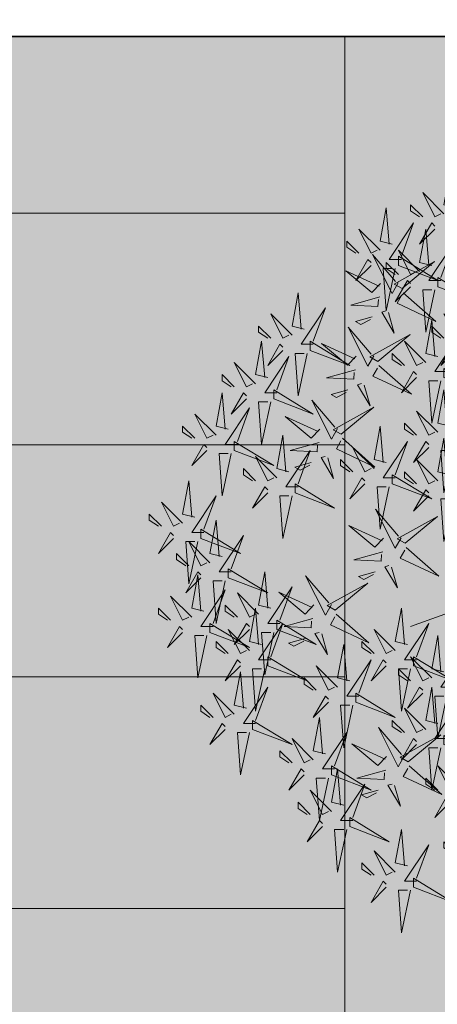
# Model space of a CAD drawing. Units: inches. Extents: x 1704 to 6393, y -157 to 1172.
# Tile 105 of 122: x 2654 to 2667, y 1002 to 1034. Entities that reach past the tile are written whole.
import ezdxf

# ---------------------------------------------------------------- set-up
doc = ezdxf.new("R2010")
doc.units = ezdxf.units.IN
doc.header["$MEASUREMENT"] = 0
for name, color, linetype, lineweight in [('A-ANNO-DIMS', 7, 'Continuous', 13), ('C-PROP', 7, 'Continuous', 35), ('L-DECK-PLNK-PATT', 250, 'Continuous', 13), ('L-HRDS', 8, 'Continuous', 18), ('L-shrub', 74, 'Continuous', 18)]:
    doc.layers.add(name, color=color, linetype=linetype, lineweight=lineweight)
doc.layers.add('L-DECK-PATT', color=35, linetype='Continuous', lineweight=13, true_color=0xa6725b)
doc.layers.add('L-HRDS-PATT', color=9, linetype='Continuous', lineweight=13, true_color=0xc5c1ba)
doc.styles.get("Standard").update_dxf_attribs({"font": 'arial.ttf'})
doc.dimstyles.get("Standard").update_dxf_attribs({"dimtxt": 6, "dimasz": 2, "dimexe": 0.18, "dimexo": 0.0625, "dimgap": 0.09, "dimtad": 0, "dimtih": 1, "dimtoh": 1, "dimdec": 1, "dimzin": 0, "dimdsep": 46, "dimlunit": 3, "dimtxsty": 'Standard', "dimblk": 'ARCHTICK', "dimcen": 0.09, "dimadec": 0, "dimazin": 0, "dimtfac": 1, "dimtdec": 1, "dimtofl": 0, "dimtmove": 0, "dimatfit": 3, "dimfxl": 1, "dimtolj": 1, "dimtzin": 0, "dimarcsym": 0})

# ---------------------------------------------------------------- blocks, each defined once
blk = doc.blocks.new('autumn shrub')
at = {"layer": 'L-shrub'}
for p, q in [((11.54, 1.92), (51.94, 98)), ((1.92, -3.84), (-38.48, 86.47)), ((-98.12, 69.17), (-107.74, 74.94)), ((0, 0), (-59.64, 40.35)), ((71.18, 17.29), (98.12, 26.9)), ((9.62, -3.84), (71.18, 17.29)), ((11.54, -5.76), (55.79, 0)), ((-5.77, -9.61), (-38.48, -19.21)), ((1.92, -13.45), (-15.39, -86.47)), ((17.31, -26.9), (25.01, -40.35)), ((-76.95, -34.59), (-126.97, -48.04)), ((-67.33, -57.64), (-80.8, -63.41)), ((46.17, -69.17), (63.49, -101.84)), ((-17.31, -122.97), (-23.09, -155.64))]:
    blk.add_line(p, q, dxfattribs=at)
for points in [[(5.77, 222.89), (11.54, 249.79), (13.47, 222.89), (7.7, 222.89)], [(-100.04, 203.68), (-94.27, 230.58), (-92.34, 203.68), (-98.12, 203.68)], [(3.85, 220.97), (-21.16, 230.58), (3.85, 215.21), (3.85, 220.97)], [(21.16, 220.97), (30.78, 230.58), (23.09, 217.13), (21.16, 219.05)], [(98.12, 194.07), (103.89, 220.97), (105.81, 194.07), (100.04, 194.07)], [(1.92, 217.13), (9.62, 217.13), (-5.77, 194.07), (1.92, 215.21)], [(15.39, 211.36), (28.86, 197.91), (21.16, 213.28), (17.31, 211.36)], [(28.86, 213.28), (36.55, 205.6), (36.55, 209.44), (30.78, 213.28)], [(-101.96, 201.75), (-126.97, 211.36), (-101.96, 195.99), (-101.96, 201.75)], [(-84.65, 201.75), (-75.03, 211.36), (-82.73, 197.91), (-84.65, 199.83)], [(-51.51, 194.97), (-55.15, 208.07), (-47.22, 194.76), (-49.84, 194.03)], [(7.7, 207.52), (15.39, 205.6), (11.54, 184.46), (9.62, 207.52)], [(46.17, 180.62), (51.94, 207.52), (53.87, 180.62), (48.1, 180.62)], [(-60.75, 182.51), (-81.34, 200.76), (-56.96, 189.22), (-59.8, 184.19)], [(-41.04, 197.9), (-30.56, 200.83), (-33.91, 202.71), (-40.09, 199.58)], [(96.19, 192.15), (71.18, 201.75), (96.19, 186.38), (96.19, 192.15)], [(113.51, 192.15), (123.13, 201.75), (115.43, 188.3), (113.51, 190.23)], [(-103.89, 197.91), (-96.19, 197.91), (-111.58, 174.85), (-103.89, 195.99)], [(-90.42, 192.15), (-76.95, 178.7), (-84.65, 194.07), (-88.5, 192.15)], [(-76.95, 194.07), (-69.26, 186.38), (-69.26, 190.23), (-75.03, 194.07)], [(-103.45, 175.76), (-107.1, 188.86), (-99.16, 175.55), (-101.78, 174.81)], [(-98.12, 188.3), (-90.42, 186.38), (-94.27, 165.25), (-96.19, 188.3)], [(-45.98, 185.23), (-27.65, 190.35), (-44.82, 191.2), (-45.03, 186.9)], [(15.39, 161.4), (21.16, 188.3), (23.09, 161.4), (17.31, 161.4)], [(44.25, 178.7), (19.24, 188.3), (44.25, 172.93), (44.25, 178.7)], [(61.56, 178.7), (71.18, 188.3), (63.49, 174.85), (61.56, 176.78)], [(94.27, 188.3), (101.96, 188.3), (86.57, 165.25), (94.27, 186.38)], [(-112.69, 163.3), (-133.28, 181.54), (-108.91, 170), (-111.74, 164.97)], [(-92.98, 178.69), (-82.5, 181.61), (-85.85, 183.5), (-92.03, 180.36)], [(-57.62, 176.33), (-53.83, 183.03), (-41.31, 158.3), (-55.94, 175.38)], [(-46.41, 176.64), (-40.96, 182.39), (-24.44, 168.66), (-45.47, 178.31)], [(107.74, 182.54), (121.2, 169.09), (113.51, 184.46), (109.66, 182.54)], [(121.2, 184.46), (128.9, 176.78), (128.9, 180.62), (123.13, 184.46)], [(138.52, 155.64), (144.29, 182.54), (146.21, 155.64), (140.44, 155.64)], [(-131.51, 152.18), (-139.33, 153.55), (-136.98, 174.91), (-133.43, 152.04)], [(-60.02, 179.89), (-80.67, 162.83), (-55, 177.06), (-60.02, 179.89)], [(42.32, 174.85), (50.02, 174.85), (34.63, 151.8), (42.32, 172.93)], [(100.04, 178.7), (107.74, 176.78), (103.89, 155.64), (101.96, 178.7)], [(-97.92, 166.01), (-79.59, 171.13), (-96.76, 171.98), (-96.98, 167.69)], [(13.47, 159.48), (-11.54, 169.09), (13.47, 153.72), (13.47, 159.48)], [(30.78, 159.48), (40.4, 169.09), (32.71, 155.64), (30.78, 157.56)], [(55.79, 169.09), (69.26, 155.64), (61.56, 171.01), (57.72, 169.09)], [(69.26, 171.01), (76.95, 163.33), (76.95, 167.17), (71.18, 171.01)], [(-184.69, 138.35), (-178.92, 165.25), (-176.99, 138.35), (-182.77, 138.35)], [(-125.08, 143), (-132.76, 142.46), (-119.03, 166.55), (-125.21, 144.92)], [(-109.56, 157.11), (-105.78, 163.82), (-93.26, 139.08), (-107.89, 156.17)], [(-98.36, 157.42), (-92.9, 163.18), (-76.38, 149.44), (-97.41, 159.1)], [(-57.28, 154.62), (-60.92, 167.72), (-52.99, 154.41), (-55.61, 153.68)], [(-46.81, 157.55), (-36.33, 160.48), (-39.68, 162.36), (-45.86, 159.22)], [(48.1, 165.25), (55.79, 163.33), (51.94, 142.19), (50.02, 165.25)], [(57.72, 140.27), (63.49, 167.17), (65.41, 140.27), (59.64, 140.27)], [(136.59, 153.72), (111.58, 163.33), (136.59, 147.95), (136.59, 153.72)], [(153.91, 153.72), (163.53, 163.33), (155.83, 149.87), (153.91, 151.8)], [(-138.92, 147.8), (-153.3, 160.27), (-144.54, 145.48), (-140.84, 147.67)], [(-111.96, 160.68), (-132.62, 143.61), (-106.94, 157.85), (-111.96, 160.68)], [(-66.52, 142.16), (-87.11, 160.4), (-62.74, 148.86), (-65.57, 143.84)], [(-152.22, 144.94), (-160.44, 152.06), (-160.16, 148.23), (-154.14, 144.8)], [(-51.75, 144.88), (-33.42, 150), (-50.59, 150.85), (-50.8, 146.55)], [(11.54, 155.64), (19.24, 155.64), (3.85, 132.58), (11.54, 153.72)], [(25.01, 149.87), (38.48, 136.42), (30.78, 151.8), (26.93, 149.87)], [(38.48, 151.8), (46.17, 144.11), (46.17, 147.95), (40.4, 151.8)], [(134.67, 149.87), (142.36, 149.87), (126.97, 126.82), (134.67, 147.95)], [(150.06, 122.97), (155.83, 149.87), (157.76, 122.97), (151.98, 122.97)], [(-186.61, 136.42), (-211.62, 146.03), (-186.61, 130.66), (-186.61, 136.42)], [(-169.3, 136.42), (-159.68, 146.03), (-167.38, 132.58), (-169.3, 134.5)], [(-126.73, 139.03), (-101.1, 131.22), (-127.13, 144.78), (-126.73, 139.03)], [(-88.06, 135.41), (-91.71, 148.51), (-83.77, 135.2), (-86.39, 134.46)], [(17.31, 146.03), (25.01, 144.11), (21.16, 122.97), (19.24, 146.03)], [(55.79, 138.35), (30.78, 147.95), (55.79, 132.58), (55.79, 138.35)], [(73.11, 138.35), (82.73, 147.95), (75.03, 134.5), (73.11, 136.42)], [(148.14, 144.11), (161.6, 130.66), (153.91, 146.03), (150.06, 144.11)], [(161.6, 146.03), (169.3, 138.35), (169.3, 142.19), (163.53, 146.03)], [(-144, 137.81), (-152.92, 127.55), (-146.19, 141.51), (-144.13, 139.73)], [(-97.3, 122.95), (-117.89, 141.19), (-93.52, 129.65), (-96.35, 124.62)], [(-65.79, 139.54), (-86.44, 122.48), (-60.77, 136.71), (-65.79, 139.54)], [(-77.59, 138.33), (-67.11, 141.26), (-70.46, 143.15), (-76.64, 140.01)], [(-63.39, 135.98), (-59.61, 142.68), (-47.08, 117.95), (-61.71, 135.03)], [(-52.18, 136.28), (-46.73, 142.04), (-30.21, 128.31), (-51.24, 137.96)], [(19.67, 127.72), (16.03, 140.82), (23.96, 127.51), (21.35, 126.78)], [(108.17, 127.72), (104.53, 140.82), (112.46, 127.51), (109.84, 126.78)], [(140.44, 140.27), (148.14, 138.35), (144.29, 117.21), (142.36, 140.27)], [(-188.54, 132.58), (-180.84, 132.58), (-196.23, 109.52), (-188.54, 130.66)], [(-157.32, 118.11), (-160.96, 131.21), (-153.03, 117.9), (-155.65, 117.17)], [(-128.51, 136.98), (-132.37, 109.74), (-136.19, 136.44), (-130.43, 136.85)], [(-82.53, 125.66), (-64.2, 130.78), (-81.37, 131.63), (-81.59, 127.34)], [(10.44, 115.26), (-10.16, 133.5), (14.22, 121.96), (11.38, 116.94)], [(30.15, 130.65), (40.62, 133.58), (37.28, 135.46), (31.09, 132.32)], [(53.87, 134.5), (61.56, 134.5), (46.17, 111.45), (53.87, 132.58)], [(98.93, 115.26), (78.34, 133.5), (102.71, 121.96), (99.88, 116.94)], [(118.64, 130.65), (129.12, 133.58), (125.77, 135.46), (119.59, 132.32)], [(-175.07, 126.82), (-161.6, 113.37), (-169.3, 128.74), (-173.15, 126.82)], [(-161.6, 128.74), (-153.91, 121.05), (-153.91, 124.9), (-159.68, 128.74)], [(-146.85, 121.04), (-136.37, 123.97), (-139.72, 125.86), (-145.9, 122.72)], [(-103.89, 101.84), (-98.12, 128.74), (-96.19, 101.84), (-101.96, 101.84)], [(59.64, 124.9), (67.33, 122.97), (63.49, 101.84), (61.56, 124.9)], [(67.33, 128.74), (80.8, 115.29), (73.11, 130.66), (69.26, 128.74)], [(78.88, 103.76), (84.65, 130.66), (86.57, 103.76), (80.8, 103.76)], [(80.8, 130.66), (88.5, 122.97), (88.5, 126.82), (82.73, 130.66)], [(148.14, 121.05), (123.13, 130.66), (148.14, 115.29), (148.14, 121.05)], [(165.45, 121.05), (175.07, 130.66), (167.38, 117.21), (165.45, 119.13)], [(-166.56, 105.65), (-187.15, 123.9), (-162.78, 112.36), (-165.61, 107.33)], [(-182.77, 122.97), (-175.07, 121.05), (-178.92, 99.92), (-180.84, 122.97)], [(-96.57, 120.33), (-117.23, 103.26), (-91.55, 117.49), (-96.57, 120.33)], [(-94.17, 116.76), (-90.39, 123.47), (-77.87, 98.73), (-92.49, 115.82)], [(-82.96, 117.07), (-77.51, 122.83), (-60.99, 109.09), (-82.02, 118.75)], [(-26.93, 94.15), (-21.16, 121.05), (-19.24, 94.15), (-25.01, 94.15)], [(25.2, 117.98), (43.54, 123.1), (26.37, 123.95), (26.15, 119.65)], [(113.7, 117.98), (132.03, 123.1), (114.86, 123.95), (114.65, 119.65)], [(200.08, 94.15), (205.85, 121.05), (207.78, 94.15), (202, 94.15)], [(-151.79, 108.37), (-133.46, 113.49), (-150.63, 114.34), (-150.84, 110.04)], [(11.17, 112.64), (-9.49, 95.58), (16.19, 109.81), (11.17, 112.64)], [(13.57, 109.08), (17.35, 115.78), (29.87, 91.05), (15.24, 108.13)], [(24.77, 109.38), (30.23, 115.14), (46.74, 101.41), (25.72, 111.06)], [(99.66, 112.64), (79.01, 95.58), (104.68, 109.81), (99.66, 112.64)], [(102.06, 109.08), (105.85, 115.78), (118.37, 91.05), (103.74, 108.13)], [(113.27, 109.38), (118.72, 115.14), (135.24, 101.41), (114.21, 111.06)], [(146.21, 117.21), (153.91, 117.21), (138.52, 94.15), (146.21, 115.29)], [(159.68, 111.45), (173.15, 98), (165.45, 113.37), (161.6, 111.45)], [(173.15, 113.37), (180.84, 105.68), (180.84, 109.52), (175.07, 113.37)], [(-184.69, 80.7), (-178.92, 107.6), (-176.99, 80.7), (-182.77, 80.7)], [(-163.43, 99.47), (-159.65, 106.17), (-147.12, 81.44), (-161.75, 98.53)], [(-105.81, 99.92), (-130.82, 109.52), (-105.81, 94.15), (-105.81, 99.92)], [(-88.5, 99.92), (-78.88, 109.52), (-86.57, 96.07), (-88.5, 98)], [(76.95, 101.84), (51.94, 111.45), (76.95, 96.07), (76.95, 101.84)], [(94.27, 101.84), (103.89, 111.45), (96.19, 98), (94.27, 99.92)], [(151.98, 107.6), (159.68, 105.68), (155.83, 84.54), (153.91, 107.6)], [(-165.83, 103.03), (-186.48, 85.97), (-160.81, 100.2), (-165.83, 103.03)], [(-152.22, 99.78), (-146.77, 105.54), (-130.25, 91.8), (-151.28, 101.45)], [(-134.24, 89.29), (-137.88, 102.39), (-129.94, 89.08), (-132.56, 88.35)], [(-80.8, 78.78), (-75.03, 105.68), (-73.11, 78.78), (-78.88, 78.78)], [(-28.86, 92.23), (-53.87, 101.84), (-28.86, 86.47), (-28.86, 92.23)], [(-11.54, 92.23), (-1.92, 101.84), (-9.62, 88.39), (-11.54, 90.31)], [(134.67, 76.86), (140.44, 103.76), (142.36, 76.86), (136.59, 76.86)], [(198.16, 92.23), (173.15, 101.84), (198.16, 86.47), (198.16, 92.23)], [(215.47, 92.23), (225.09, 101.84), (217.4, 88.39), (215.47, 90.31)], [(-143.47, 76.83), (-164.07, 95.07), (-139.69, 83.53), (-142.53, 78.51)], [(-123.76, 92.22), (-113.29, 95.15), (-116.63, 97.03), (-122.82, 93.89)], [(-107.74, 96.07), (-100.04, 96.07), (-115.43, 73.02), (-107.74, 94.15)], [(75.03, 98), (82.73, 98), (67.33, 74.94), (75.03, 96.07)], [(75.03, 71.09), (80.8, 98), (82.73, 71.09), (76.95, 71.09)], [(88.5, 92.23), (101.96, 78.78), (94.27, 94.15), (90.42, 92.23)], [(101.96, 94.15), (109.66, 86.47), (109.66, 90.31), (103.89, 94.15)], [(-186.61, 78.78), (-211.62, 88.39), (-186.61, 73.02), (-186.61, 78.78)], [(-169.3, 78.78), (-159.68, 88.39), (-167.38, 74.94), (-169.3, 76.86)], [(-94.27, 90.31), (-80.8, 76.86), (-88.5, 92.23), (-92.34, 90.31)], [(-80.8, 92.23), (-73.11, 84.54), (-73.11, 88.39), (-78.88, 92.23)], [(-30.78, 88.39), (-23.09, 88.39), (-38.48, 65.33), (-30.78, 86.47)], [(80.8, 88.39), (88.5, 86.47), (84.65, 65.33), (82.73, 88.39)], [(196.23, 88.39), (203.93, 88.39), (188.54, 65.33), (196.23, 86.47)], [(-128.7, 79.55), (-110.37, 84.67), (-127.54, 85.52), (-127.76, 81.22)], [(-82.73, 76.86), (-107.74, 86.47), (-82.73, 71.09), (-82.73, 76.86)], [(-101.96, 86.47), (-94.27, 84.54), (-98.12, 63.41), (-100.04, 86.47)], [(-65.41, 76.86), (-55.79, 86.47), (-63.49, 73.02), (-65.41, 74.94)], [(-17.31, 82.62), (-3.85, 69.17), (-11.54, 84.54), (-15.39, 82.62)], [(-3.85, 84.54), (3.85, 76.86), (3.85, 80.7), (-1.92, 84.54)], [(44.25, 57.64), (50.02, 84.54), (51.94, 57.64), (46.17, 57.64)], [(132.75, 74.94), (107.74, 84.54), (132.75, 69.17), (132.75, 74.94)], [(150.06, 74.94), (159.68, 84.54), (151.98, 71.09), (150.06, 73.02)], [(209.7, 82.62), (223.17, 69.17), (215.47, 84.54), (211.62, 82.62)], [(223.17, 84.54), (230.86, 76.86), (230.86, 80.7), (225.09, 84.54)], [(-188.54, 74.94), (-180.84, 74.94), (-196.23, 51.88), (-188.54, 73.02)], [(-140.34, 70.65), (-136.56, 77.35), (-124.04, 52.62), (-138.67, 69.7)], [(-129.14, 70.95), (-123.68, 76.71), (-107.16, 62.98), (-128.19, 72.63)], [(-25.01, 78.78), (-17.31, 76.86), (-21.16, 55.72), (-23.09, 78.78)], [(42.76, 62.39), (39.12, 75.49), (47.05, 62.18), (44.43, 61.45)], [(73.11, 69.17), (48.1, 78.78), (73.11, 63.41), (73.11, 69.17)], [(90.42, 69.17), (100.04, 78.78), (92.34, 65.33), (90.42, 67.25)], [(98.12, 53.8), (103.89, 80.7), (105.81, 53.8), (100.04, 53.8)], [(190.46, 53.8), (196.23, 80.7), (198.16, 53.8), (192.39, 53.8)], [(202, 78.78), (209.7, 76.86), (205.85, 55.72), (203.93, 78.78)], [(-175.07, 69.17), (-161.6, 55.72), (-169.3, 71.09), (-173.15, 69.17)], [(-142.74, 74.21), (-163.4, 57.15), (-137.72, 71.38), (-142.74, 74.21)], [(-161.6, 71.09), (-153.91, 63.41), (-153.91, 67.25), (-159.68, 71.09)], [(-84.65, 73.02), (-76.95, 73.02), (-92.34, 49.96), (-84.65, 71.09)], [(-71.18, 67.25), (-57.72, 53.8), (-65.41, 69.17), (-69.26, 67.25)], [(-57.72, 69.17), (-50.02, 61.49), (-50.02, 65.33), (-55.79, 69.17)], [(53.23, 65.32), (63.71, 68.25), (60.36, 70.13), (54.18, 66.99)], [(130.82, 71.09), (138.52, 71.09), (123.13, 48.04), (130.82, 69.17)], [(-182.77, 65.33), (-175.07, 63.41), (-178.92, 42.27), (-180.84, 65.33)], [(-161.17, 52.78), (-164.81, 65.88), (-156.88, 52.57), (-159.5, 51.84)], [(-78.88, 63.41), (-71.18, 61.49), (-75.03, 40.35), (-76.95, 63.41)], [(33.52, 49.93), (12.93, 68.17), (37.3, 56.63), (34.47, 51.61)], [(42.32, 55.72), (17.31, 65.33), (42.32, 49.96), (42.32, 55.72)], [(59.64, 55.72), (69.26, 65.33), (61.56, 51.88), (59.64, 53.8)], [(71.18, 65.33), (78.88, 65.33), (63.49, 42.27), (71.18, 63.41)], [(144.29, 65.33), (157.76, 51.88), (150.06, 67.25), (146.21, 65.33)], [(157.76, 67.25), (165.45, 59.57), (165.45, 63.41), (159.68, 67.25)], [(-228.94, 32.67), (-223.17, 59.57), (-221.24, 32.67), (-227.01, 32.67)], [(-170.4, 40.32), (-191, 58.57), (-166.62, 47.03), (-169.46, 42)], [(-150.69, 55.71), (-140.22, 58.64), (-143.57, 60.53), (-149.75, 57.39)], [(48.29, 52.64), (66.62, 57.77), (49.45, 58.62), (49.24, 54.32)], [(96.19, 51.88), (71.18, 61.49), (96.19, 46.12), (96.19, 51.88)], [(84.65, 59.57), (98.12, 46.12), (90.42, 61.49), (86.57, 59.57)], [(98.12, 61.49), (105.81, 53.8), (105.81, 57.64), (100.04, 61.49)], [(113.51, 51.88), (123.13, 61.49), (115.43, 48.04), (113.51, 49.96)], [(136.59, 61.49), (144.29, 59.57), (140.44, 38.43), (138.52, 61.49)], [(188.54, 51.88), (163.53, 61.49), (188.54, 46.12), (188.54, 51.88)], [(184.69, 30.74), (190.46, 57.64), (192.39, 30.74), (186.61, 30.74)], [(205.85, 51.88), (215.47, 61.49), (207.78, 48.04), (205.85, 49.96)], [(227.01, 32.67), (232.79, 59.57), (234.71, 32.67), (228.94, 32.67)], [(40.4, 51.88), (48.1, 51.88), (32.71, 28.82), (40.4, 49.96)], [(36.65, 43.75), (40.43, 50.45), (52.96, 25.72), (38.33, 42.8)], [(76.95, 55.72), (84.65, 53.8), (80.8, 32.67), (78.88, 55.72)], [(-155.64, 43.04), (-137.31, 48.16), (-154.48, 49.01), (-154.69, 44.71)], [(34.25, 47.31), (13.6, 30.25), (39.27, 44.48), (34.25, 47.31)], [(47.86, 44.05), (53.31, 49.81), (69.83, 36.08), (48.8, 45.73)], [(53.87, 46.12), (67.33, 32.67), (59.64, 48.04), (55.79, 46.12)], [(67.33, 48.04), (75.03, 40.35), (75.03, 44.19), (69.26, 48.04)], [(94.27, 48.04), (101.96, 48.04), (86.57, 24.98), (94.27, 46.12)], [(107.74, 42.27), (121.2, 28.82), (113.51, 44.19), (109.66, 42.27)], [(121.2, 44.19), (128.9, 36.51), (128.9, 40.35), (123.13, 44.19)], [(154.34, 31.65), (150.7, 44.75), (158.63, 31.44), (156.02, 30.7)], [(186.61, 48.04), (194.31, 48.04), (178.92, 24.98), (186.61, 46.12)], [(200.08, 42.27), (213.55, 28.82), (205.85, 44.19), (202, 42.27)], [(213.55, 44.19), (221.24, 36.51), (221.24, 40.35), (215.47, 44.19)], [(-230.86, 30.74), (-255.87, 40.35), (-230.86, 24.98), (-230.86, 30.74)], [(-213.55, 30.74), (-203.93, 40.35), (-211.62, 26.9), (-213.55, 28.82)], [(-169.68, 37.7), (-190.33, 20.64), (-164.66, 34.87), (-169.68, 37.7)], [(-167.27, 34.14), (-163.49, 40.84), (-150.97, 16.11), (-165.6, 33.2)], [(-156.07, 34.45), (-150.62, 40.21), (-134.1, 26.47), (-155.13, 36.12)], [(-76.52, 29.73), (-80.16, 42.83), (-72.23, 29.51), (-74.85, 28.78)], [(-66.05, 32.65), (-55.57, 35.58), (-58.92, 37.47), (-65.1, 34.33)], [(46.17, 42.27), (53.87, 40.35), (50.02, 19.21), (48.1, 42.27)], [(100.04, 38.43), (107.74, 36.51), (103.89, 15.37), (101.96, 38.43)], [(145.11, 19.19), (124.51, 37.43), (148.89, 25.89), (146.05, 20.86)], [(182.77, 28.82), (157.76, 38.43), (182.77, 23.06), (182.77, 28.82)], [(164.82, 34.57), (175.29, 37.5), (171.94, 39.39), (165.76, 36.25)], [(192.39, 38.43), (200.08, 36.51), (196.23, 15.37), (194.31, 38.43)], [(225.09, 30.74), (200.08, 40.35), (225.09, 24.98), (225.09, 30.74)], [(200.08, 28.82), (209.7, 38.43), (202, 24.98), (200.08, 26.9)], [(242.41, 30.74), (252.02, 40.35), (244.33, 26.9), (242.41, 28.82)], [(-85.76, 17.27), (-106.35, 35.51), (-81.97, 23.97), (-84.81, 18.94)], [(-232.79, 26.9), (-225.09, 26.9), (-240.48, 3.84), (-232.79, 24.98)], [(-70.99, 19.98), (-52.66, 25.1), (-69.83, 25.95), (-70.04, 21.66)], [(159.87, 21.9), (178.21, 27.02), (161.04, 27.87), (160.82, 23.58)], [(180.84, 24.98), (188.54, 24.98), (173.15, 1.92), (180.84, 23.06)], [(223.17, 26.9), (230.86, 26.9), (215.47, 3.84), (223.17, 24.98)], [(215.47, -1.92), (221.24, 24.98), (223.17, -1.92), (217.4, -1.92)], [(-219.32, 21.14), (-205.85, 7.69), (-213.55, 23.06), (-217.4, 21.14)], [(-213.55, -3.84), (-207.78, 23.06), (-205.85, -3.84), (-211.62, -3.84)], [(-205.85, 23.06), (-198.16, 15.37), (-198.16, 19.21), (-203.93, 23.06)], [(-161.6, -7.69), (-155.83, 19.21), (-153.91, -7.69), (-159.68, -7.69)], [(-96.19, -5.76), (-90.42, 21.14), (-88.5, -5.76), (-94.27, -5.76)], [(-57.72, -3.84), (-51.94, 23.06), (-50.02, -3.84), (-55.79, -3.84)], [(148.24, 13), (152.02, 19.71), (164.54, -5.03), (149.91, 12.06)], [(159.44, 13.31), (164.89, 19.07), (181.41, 5.33), (160.39, 14.99)], [(194.31, 19.21), (207.78, 5.76), (200.08, 21.14), (196.23, 19.21)], [(207.78, 21.14), (215.47, 13.45), (215.47, 17.29), (209.7, 21.14)], [(236.63, 21.14), (250.1, 7.69), (242.41, 23.06), (238.56, 21.14)], [(250.1, 23.06), (257.8, 15.37), (257.8, 19.21), (252.02, 23.06)], [(-227.01, 17.29), (-219.32, 15.37), (-223.17, -5.76), (-225.09, 17.29)], [(-85.03, 14.65), (-105.68, -2.42), (-80.01, 11.81), (-85.03, 14.65)], [(-82.63, 11.08), (-78.84, 17.78), (-66.32, -6.95), (-80.95, 10.14)], [(-71.42, 11.39), (-65.97, 17.15), (-49.45, 3.41), (-70.48, 13.06)], [(34.63, -9.61), (40.4, 17.29), (42.32, -9.61), (36.55, -9.61)], [(145.83, 16.57), (125.18, -0.5), (150.86, 13.74), (145.83, 16.57)], [(186.61, 15.37), (194.31, 13.45), (190.46, -7.69), (188.54, 15.37)], [(228.94, 17.29), (236.63, 15.37), (232.79, -5.76), (230.86, 17.29)], [(-215.47, -5.76), (-240.48, 3.84), (-215.47, -11.53), (-215.47, -5.76)], [(-198.16, -5.76), (-188.54, 3.84), (-196.23, -9.61), (-198.16, -7.69)], [(-163.53, -9.61), (-188.54, 0), (-163.53, -15.37), (-163.53, -9.61)], [(-146.21, -9.61), (-136.59, 0), (-144.29, -13.45), (-146.21, -11.53)], [(-98.12, -7.69), (-123.13, 1.92), (-98.12, -13.45), (-98.12, -7.69)], [(-59.64, -5.76), (-84.65, 3.84), (-59.64, -11.53), (-59.64, -5.76)], [(-80.8, -7.69), (-71.18, 1.92), (-78.88, -11.53), (-80.8, -9.61)], [(-42.32, -5.76), (-32.71, 3.84), (-40.4, -9.61), (-42.32, -7.69)], [(110.09, -10.62), (106.45, 2.47), (114.39, -10.84), (111.77, -11.57)], [(213.55, -3.84), (188.54, 5.76), (213.55, -9.61), (213.55, -3.84)], [(230.86, -3.84), (240.48, 5.76), (232.79, -7.69), (230.86, -5.76)], [(232.79, -26.9), (238.56, 0), (240.48, -26.9), (234.71, -26.9)], [(32.71, -11.53), (7.7, -1.92), (32.71, -17.29), (32.71, -11.53)], [(50.02, -11.53), (59.64, -1.92), (51.94, -15.37), (50.02, -13.45)], [(100.86, -23.09), (80.26, -4.84), (104.64, -16.38), (101.8, -21.41)], [(120.57, -7.7), (131.04, -4.77), (127.7, -2.88), (121.51, -6.02)], [(-217.4, -9.61), (-209.7, -9.61), (-225.09, -32.67), (-217.4, -11.53)], [(-100.04, -11.53), (-92.34, -11.53), (-107.74, -34.59), (-100.04, -13.45)], [(-61.56, -9.61), (-53.87, -9.61), (-69.26, -32.67), (-61.56, -11.53)], [(211.62, -7.69), (219.32, -7.69), (203.93, -30.74), (211.62, -9.61)], [(225.09, -13.45), (238.56, -26.9), (230.86, -11.53), (227.01, -13.45)], [(238.56, -11.53), (246.25, -19.21), (246.25, -15.37), (240.48, -11.53)], [(-203.93, -15.37), (-190.46, -28.82), (-198.16, -13.45), (-202, -15.37)], [(-190.46, -13.45), (-182.77, -21.14), (-182.77, -17.29), (-188.54, -13.45)], [(-165.45, -13.45), (-157.76, -13.45), (-173.15, -36.51), (-165.45, -15.37)], [(-151.98, -19.21), (-138.52, -32.67), (-146.21, -17.29), (-150.06, -19.21)], [(-138.52, -17.29), (-130.82, -24.98), (-130.82, -21.14), (-136.59, -17.29)], [(-86.57, -17.29), (-73.11, -30.74), (-80.8, -15.37), (-84.65, -17.29)], [(-78.88, -44.19), (-73.11, -17.29), (-71.18, -44.19), (-76.95, -44.19)], [(-73.11, -15.37), (-65.41, -23.06), (-65.41, -19.21), (-71.18, -15.37)], [(-48.1, -15.37), (-34.63, -28.82), (-42.32, -13.45), (-46.17, -15.37)], [(-34.63, -13.45), (-26.93, -21.14), (-26.93, -17.29), (-32.71, -13.45)], [(30.78, -15.37), (38.48, -15.37), (23.09, -38.43), (30.78, -17.29)], [(115.63, -20.37), (133.96, -15.25), (116.79, -14.4), (116.57, -18.7)], [(217.4, -17.29), (225.09, -19.21), (221.24, -40.35), (219.32, -17.29)], [(-228.94, -48.04), (-223.17, -21.14), (-221.24, -48.04), (-227.01, -48.04)], [(-211.62, -19.21), (-203.93, -21.14), (-207.78, -42.27), (-209.7, -19.21)], [(-159.68, -23.06), (-151.98, -24.98), (-155.83, -46.12), (-157.76, -23.06)], [(-94.27, -21.14), (-86.57, -23.06), (-90.42, -44.19), (-92.34, -21.14)], [(-55.79, -19.21), (-48.1, -21.14), (-51.94, -42.27), (-53.87, -19.21)], [(44.25, -21.14), (57.72, -34.59), (50.02, -19.21), (46.17, -21.14)], [(57.72, -19.21), (65.41, -26.9), (65.41, -23.06), (59.64, -19.21)], [(103.99, -29.27), (107.77, -22.57), (120.29, -47.3), (105.66, -30.21)], [(115.19, -28.96), (120.65, -23.2), (137.17, -36.94), (116.14, -27.29)], [(230.86, -28.82), (205.85, -19.21), (230.86, -34.59), (230.86, -28.82)], [(248.18, -28.82), (257.8, -19.21), (250.1, -32.67), (248.18, -30.74)], [(36.55, -24.98), (44.25, -26.9), (40.4, -48.04), (38.48, -24.98)], [(71.18, -53.8), (76.95, -26.9), (78.88, -53.8), (73.11, -53.8)], [(101.59, -25.71), (80.93, -42.77), (106.61, -28.54), (101.59, -25.71)], [(173.15, -55.72), (178.92, -28.82), (180.84, -55.72), (175.07, -55.72)], [(-80.8, -46.12), (-105.81, -36.51), (-80.8, -51.88), (-80.8, -46.12)], [(-63.49, -46.12), (-53.87, -36.51), (-61.56, -49.96), (-63.49, -48.04)], [(40.4, -59.57), (46.17, -32.67), (48.1, -59.57), (42.32, -59.57)], [(111.58, -61.49), (117.35, -34.59), (119.28, -61.49), (113.51, -61.49)], [(228.94, -32.67), (236.63, -32.67), (221.24, -55.72), (228.94, -34.59)], [(242.41, -38.43), (255.87, -51.88), (248.18, -36.51), (244.33, -38.43)], [(255.87, -36.51), (263.57, -44.19), (263.57, -40.35), (257.8, -36.51)], [(-230.86, -49.96), (-255.87, -40.35), (-230.86, -55.72), (-230.86, -49.96)], [(-213.55, -49.96), (-203.93, -40.35), (-211.62, -53.8), (-213.55, -51.88)], [(-188.54, -69.17), (-182.77, -42.27), (-180.84, -69.17), (-186.61, -69.17)], [(-141.93, -52.9), (-145.57, -39.8), (-137.64, -53.11), (-140.26, -53.84)], [(234.71, -42.27), (242.41, -44.19), (238.56, -65.33), (236.63, -42.27)], [(-151.17, -65.36), (-171.76, -47.11), (-147.39, -58.66), (-150.22, -63.68)], [(-131.46, -49.97), (-120.98, -47.04), (-124.33, -45.16), (-130.51, -48.29)], [(69.26, -55.72), (44.25, -46.12), (69.26, -61.49), (69.26, -55.72)], [(86.57, -55.72), (96.19, -46.12), (88.5, -59.57), (86.57, -57.64)], [(171.22, -57.64), (146.21, -48.04), (171.22, -63.41), (171.22, -57.64)], [(188.54, -57.64), (198.16, -48.04), (190.46, -61.49), (188.54, -59.57)], [(-232.79, -53.8), (-225.09, -53.8), (-240.48, -76.86), (-232.79, -55.72)], [(-82.73, -49.96), (-75.03, -49.96), (-90.42, -73.02), (-82.73, -51.88)], [(-76.95, -80.7), (-71.18, -53.8), (-69.26, -80.7), (-75.03, -80.7)], [(-69.26, -55.72), (-55.79, -69.17), (-63.49, -53.8), (-67.33, -55.72)], [(-55.79, -53.8), (-48.1, -61.49), (-48.1, -57.64), (-53.87, -53.8)], [(-30.78, -76.86), (-25.01, -49.96), (-23.09, -76.86), (-28.86, -76.86)], [(38.48, -61.49), (13.47, -51.88), (38.48, -67.25), (38.48, -61.49)], [(55.79, -61.49), (65.41, -51.88), (57.72, -65.33), (55.79, -63.41)], [(109.66, -63.41), (84.65, -53.8), (109.66, -69.17), (109.66, -63.41)], [(126.97, -63.41), (136.59, -53.8), (128.9, -67.25), (126.97, -65.33)], [(211.62, -82.62), (217.4, -55.72), (219.32, -82.62), (213.55, -82.62)], [(-219.32, -59.57), (-205.85, -73.02), (-213.55, -57.64), (-217.4, -59.57)], [(-190.46, -71.09), (-215.47, -61.49), (-190.46, -76.86), (-190.46, -71.09)], [(-205.85, -57.64), (-198.16, -65.33), (-198.16, -61.49), (-203.93, -57.64)], [(-173.15, -71.09), (-163.53, -61.49), (-171.22, -74.94), (-173.15, -73.02)], [(-136.4, -62.64), (-118.07, -57.52), (-135.24, -56.67), (-135.45, -60.97)], [(-76.95, -59.57), (-69.26, -61.49), (-73.11, -82.62), (-75.03, -59.57)], [(67.33, -59.57), (75.03, -59.57), (59.64, -82.62), (67.33, -61.49)], [(71.18, -84.54), (76.95, -57.64), (78.88, -84.54), (73.11, -84.54)], [(169.3, -61.49), (176.99, -61.49), (161.6, -84.54), (169.3, -63.41)], [(-227.01, -63.41), (-219.32, -65.33), (-223.17, -86.47), (-225.09, -63.41)], [(-150.44, -67.98), (-171.09, -85.04), (-145.42, -70.81), (-150.44, -67.98)], [(-148.04, -71.54), (-144.26, -64.84), (-131.73, -89.57), (-146.36, -72.49)], [(-136.83, -71.23), (-131.38, -65.48), (-114.86, -79.21), (-135.89, -69.56)], [(36.55, -65.33), (44.25, -65.33), (28.86, -88.39), (36.55, -67.25)], [(80.8, -65.33), (94.27, -78.78), (86.57, -63.41), (82.73, -65.33)], [(94.27, -63.41), (101.96, -71.09), (101.96, -67.25), (96.19, -63.41)], [(107.74, -67.25), (115.43, -67.25), (100.04, -90.31), (107.74, -69.17)], [(150.49, -79.8), (146.85, -66.7), (154.79, -80.01), (152.17, -80.74)], [(182.77, -67.25), (196.23, -80.7), (188.54, -65.33), (184.69, -67.25)], [(196.23, -65.33), (203.93, -73.02), (203.93, -69.17), (198.16, -65.33)], [(-142.36, -96.07), (-136.59, -69.17), (-134.67, -96.07), (-140.44, -96.07)], [(-78.88, -82.62), (-103.89, -73.02), (-78.88, -88.39), (-78.88, -82.62)], [(-61.56, -82.62), (-51.94, -73.02), (-59.64, -86.47), (-61.56, -84.54)], [(-32.71, -78.78), (-57.72, -69.17), (-32.71, -84.54), (-32.71, -78.78)], [(-15.39, -78.78), (-5.77, -69.17), (-13.47, -82.62), (-15.39, -80.7)], [(50.02, -71.09), (63.49, -84.54), (55.79, -69.17), (51.94, -71.09)], [(63.49, -69.17), (71.18, -76.86), (71.18, -73.02), (65.41, -69.17)], [(73.11, -69.17), (80.8, -71.09), (76.95, -92.23), (75.03, -69.17)], [(141.26, -92.26), (120.66, -74.02), (145.04, -85.56), (142.2, -90.58)], [(121.2, -73.02), (134.67, -86.47), (126.97, -71.09), (123.13, -73.02)], [(134.67, -71.09), (142.36, -78.78), (142.36, -74.94), (136.59, -71.09)], [(160.97, -76.87), (171.44, -73.94), (168.1, -72.06), (161.91, -75.19)], [(175.07, -71.09), (182.77, -73.02), (178.92, -94.15), (176.99, -71.09)], [(-192.39, -74.94), (-184.69, -74.94), (-200.08, -98), (-192.39, -76.86)], [(-178.92, -80.7), (-165.45, -94.15), (-173.15, -78.78), (-176.99, -80.7)], [(-165.45, -78.78), (-157.76, -86.47), (-157.76, -82.62), (-163.53, -78.78)], [(42.32, -74.94), (50.02, -76.86), (46.17, -98), (44.25, -74.94)], [(69.26, -86.47), (44.25, -76.86), (69.26, -92.23), (69.26, -86.47)], [(86.57, -86.47), (96.19, -76.86), (88.5, -90.31), (86.57, -88.39)], [(113.51, -76.86), (121.2, -78.78), (117.35, -99.92), (115.43, -76.86)], [(209.7, -84.54), (184.69, -74.94), (209.7, -90.31), (209.7, -84.54)], [(227.01, -84.54), (236.63, -74.94), (228.94, -88.39), (227.01, -86.47)], [(-186.61, -84.54), (-178.92, -86.47), (-182.77, -107.6), (-184.69, -84.54)], [(-80.8, -86.47), (-73.11, -86.47), (-88.5, -109.52), (-80.8, -88.39)], [(-34.63, -82.62), (-26.93, -82.62), (-42.32, -105.68), (-34.63, -84.54)], [(-21.16, -88.39), (-7.7, -101.84), (-15.39, -86.47), (-19.24, -88.39)], [(-7.7, -86.47), (0, -94.15), (0, -90.31), (-5.77, -86.47)], [(156.03, -89.54), (174.36, -84.42), (157.19, -83.57), (156.97, -87.87)], [(-144.29, -98), (-169.3, -88.39), (-144.29, -103.76), (-144.29, -98)], [(-126.97, -98), (-117.35, -88.39), (-125.05, -101.84), (-126.97, -99.92)], [(-67.33, -92.23), (-53.87, -105.68), (-61.56, -90.31), (-65.41, -92.23)], [(-53.87, -90.31), (-46.17, -98), (-46.17, -94.15), (-51.94, -90.31)], [(-28.86, -92.23), (-21.16, -94.15), (-25.01, -115.29), (-26.93, -92.23)], [(67.33, -90.31), (75.03, -90.31), (59.64, -113.37), (67.33, -92.23)], [(144.39, -98.44), (148.17, -91.74), (160.69, -116.47), (146.06, -99.39)], [(155.59, -98.13), (161.05, -92.38), (177.57, -106.11), (156.54, -96.46)], [(186.61, -115.29), (192.39, -88.39), (194.31, -115.29), (188.54, -115.29)], [(207.78, -88.39), (215.47, -88.39), (200.08, -111.45), (207.78, -90.31)], [(221.24, -94.15), (234.71, -107.6), (227.01, -92.23), (223.17, -94.15)], [(234.71, -92.23), (242.41, -99.92), (242.41, -96.07), (236.63, -92.23)], [(-75.03, -96.07), (-67.33, -98), (-71.18, -119.13), (-73.11, -96.07)], [(80.8, -96.07), (94.27, -109.52), (86.57, -94.15), (82.73, -96.07)], [(94.27, -94.15), (101.96, -101.84), (101.96, -98), (96.19, -94.15)], [(141.99, -94.88), (121.33, -111.94), (147.01, -97.71), (141.99, -94.88)], [(213.55, -98), (221.24, -99.92), (217.4, -121.05), (215.47, -98)], [(-146.21, -101.84), (-138.52, -101.84), (-153.91, -124.9), (-146.21, -103.76)], [(-132.75, -107.6), (-119.28, -121.05), (-126.97, -105.68), (-130.82, -107.6)], [(-119.28, -105.68), (-111.58, -113.37), (-111.58, -109.52), (-117.35, -105.68)], [(-88.06, -118.23), (-91.71, -105.13), (-83.77, -118.44), (-86.39, -119.17)], [(10.05, -118.23), (6.41, -105.13), (14.35, -118.44), (11.73, -119.17)], [(73.11, -99.92), (80.8, -101.84), (76.95, -122.97), (75.03, -99.92)], [(78.88, -128.74), (84.65, -101.84), (86.57, -128.74), (80.8, -128.74)], [(-140.44, -111.45), (-132.75, -113.37), (-136.59, -134.5), (-138.52, -111.45)], [(-130.82, -134.5), (-125.05, -107.6), (-123.13, -134.5), (-128.9, -134.5)], [(-77.59, -115.3), (-67.11, -112.37), (-70.46, -110.49), (-76.64, -113.62)], [(20.53, -115.3), (31, -112.37), (27.66, -110.49), (21.47, -113.62)], [(184.69, -117.21), (159.68, -107.6), (184.69, -122.97), (184.69, -117.21)], [(202, -117.21), (211.62, -107.6), (203.93, -121.05), (202, -119.13)], [(-182.77, -142.19), (-176.99, -115.29), (-175.07, -142.19), (-180.84, -142.19)], [(-97.3, -130.69), (-117.89, -112.44), (-93.52, -123.99), (-96.35, -129.01)], [(0.82, -130.69), (-19.78, -112.44), (4.6, -123.99), (1.76, -129.01)], [(127.41, -125.91), (123.77, -112.81), (131.7, -126.12), (129.08, -126.86)], [(137.88, -122.99), (148.36, -120.06), (145.01, -118.17), (138.83, -121.31)], [(-82.53, -127.97), (-64.2, -122.85), (-81.37, -122), (-81.59, -126.3)], [(15.59, -127.97), (33.92, -122.85), (16.75, -122), (16.53, -126.3)], [(76.95, -130.66), (51.94, -121.05), (76.95, -136.42), (76.95, -130.66)], [(53.87, -146.03), (59.64, -119.13), (61.56, -146.03), (55.79, -146.03)], [(94.27, -130.66), (103.89, -121.05), (96.19, -134.5), (94.27, -132.58)], [(118.17, -138.37), (97.58, -120.13), (121.95, -131.67), (119.12, -136.7)], [(163.53, -146.03), (169.3, -119.13), (171.22, -146.03), (165.45, -146.03)], [(182.77, -121.05), (190.46, -121.05), (175.07, -144.11), (182.77, -122.97)], [(-132.75, -136.42), (-157.76, -126.82), (-132.75, -142.19), (-132.75, -136.42)], [(-115.43, -136.42), (-105.81, -126.82), (-113.51, -140.27), (-115.43, -138.35)], [(-94.17, -136.87), (-90.39, -130.17), (-77.87, -154.9), (-92.49, -137.82)], [(-82.96, -136.56), (-77.51, -130.81), (-60.99, -144.54), (-82.02, -134.89)], [(-82.73, -157.56), (-76.95, -130.66), (-75.03, -157.56), (-80.8, -157.56)], [(3.95, -136.87), (7.73, -130.17), (20.25, -154.9), (5.62, -137.82)], [(15.15, -136.56), (20.61, -130.81), (37.13, -144.54), (16.1, -134.89)], [(132.94, -135.66), (151.27, -130.54), (134.1, -129.69), (133.89, -133.98)], [(188.54, -130.66), (196.23, -132.58), (192.39, -153.72), (190.46, -130.66)], [(196.23, -126.82), (209.7, -140.27), (202, -124.9), (198.16, -126.82)], [(209.7, -124.9), (217.4, -132.58), (217.4, -128.74), (211.62, -124.9)], [(-184.69, -144.11), (-209.7, -134.5), (-184.69, -149.87), (-184.69, -144.11)], [(-167.38, -144.11), (-157.76, -134.5), (-165.45, -147.95), (-167.38, -146.03)], [(-96.57, -133.31), (-117.23, -150.37), (-91.55, -136.14), (-96.57, -133.31)], [(-39.97, -145.13), (-43.61, -132.03), (-35.67, -145.34), (-38.29, -146.07)], [(1.55, -133.31), (-19.11, -150.37), (6.57, -136.14), (1.55, -133.31)], [(75.03, -134.5), (82.73, -134.5), (67.33, -157.56), (75.03, -136.42)], [(-134.67, -140.27), (-126.97, -140.27), (-142.36, -163.33), (-134.67, -142.19)], [(-49.2, -157.59), (-69.8, -139.35), (-45.42, -150.89), (-48.26, -155.91)], [(-29.49, -142.2), (-19.02, -139.27), (-22.36, -137.39), (-28.55, -140.52)], [(51.94, -147.95), (26.93, -138.35), (51.94, -153.72), (51.94, -147.95)], [(69.26, -147.95), (78.88, -138.35), (71.18, -151.8), (69.26, -149.87)], [(88.5, -140.27), (101.96, -153.72), (94.27, -138.35), (90.42, -140.27)], [(118.9, -140.99), (98.25, -158.06), (123.92, -143.83), (118.9, -140.99)], [(101.96, -138.35), (109.66, -146.03), (109.66, -142.19), (103.89, -138.35)], [(121.3, -144.56), (125.08, -137.85), (137.61, -162.59), (122.98, -145.5)], [(132.51, -144.25), (137.96, -138.49), (154.48, -152.23), (133.45, -142.57)], [(161.6, -147.95), (136.59, -138.35), (161.6, -153.72), (161.6, -147.95)], [(178.92, -147.95), (188.54, -138.35), (180.84, -151.8), (178.92, -149.87)], [(-186.61, -147.95), (-178.92, -147.95), (-194.31, -171.01), (-186.61, -149.87)], [(-121.2, -146.03), (-107.74, -159.48), (-115.43, -144.11), (-119.28, -146.03)], [(-107.74, -144.11), (-100.04, -151.8), (-100.04, -147.95), (-105.81, -144.11)], [(-34.43, -154.87), (-16.1, -149.75), (-33.27, -148.9), (-33.49, -153.2)], [(80.8, -144.11), (88.5, -146.03), (84.65, -167.17), (82.73, -144.11)], [(-173.15, -153.72), (-159.68, -167.17), (-167.38, -151.8), (-171.22, -153.72)], [(-159.68, -151.8), (-151.98, -159.48), (-151.98, -155.64), (-157.76, -151.8)], [(-128.9, -149.87), (-121.2, -151.8), (-125.05, -172.93), (-126.97, -149.87)], [(-84.65, -159.48), (-109.66, -149.87), (-84.65, -165.25), (-84.65, -159.48)], [(-67.33, -159.48), (-57.72, -149.87), (-65.41, -163.33), (-67.33, -161.4)], [(-36.55, -176.78), (-30.78, -149.87), (-28.86, -176.78), (-34.63, -176.78)], [(50.02, -151.8), (57.72, -151.8), (42.32, -174.85), (50.02, -153.72)], [(63.49, -157.56), (76.95, -171.01), (69.26, -155.64), (65.41, -157.56)], [(76.95, -155.64), (84.65, -163.33), (84.65, -159.48), (78.88, -155.64)], [(159.68, -151.8), (167.38, -151.8), (151.98, -174.85), (159.68, -153.72)], [(173.15, -157.56), (186.61, -171.01), (178.92, -155.64), (175.07, -157.56)], [(186.61, -155.64), (194.31, -163.33), (194.31, -159.48), (188.54, -155.64)], [(-180.84, -157.56), (-173.15, -159.48), (-176.99, -180.62), (-178.92, -157.56)], [(-48.47, -160.21), (-69.13, -177.27), (-43.45, -163.04), (-48.47, -160.21)], [(-46.07, -163.77), (-42.29, -157.07), (-29.77, -181.8), (-44.4, -164.72)], [(-34.87, -163.46), (-29.41, -157.71), (-12.89, -171.44), (-33.92, -161.79)], [(9.62, -184.46), (15.39, -157.56), (17.31, -184.46), (11.54, -184.46)], [(55.79, -161.4), (63.49, -163.33), (59.64, -184.46), (57.72, -161.4)], [(82.73, -186.38), (88.5, -159.48), (90.42, -186.38), (84.65, -186.38)], [(112.02, -172.03), (108.37, -158.93), (116.31, -172.24), (113.69, -172.97)], [(165.45, -161.4), (173.15, -163.33), (169.3, -184.46), (167.38, -161.4)], [(-103.89, -190.23), (-98.12, -163.33), (-96.19, -190.23), (-101.96, -190.23)], [(-86.57, -163.33), (-78.88, -163.33), (-94.27, -186.38), (-86.57, -165.25)], [(-73.11, -169.09), (-59.64, -182.54), (-67.33, -167.17), (-71.18, -169.09)], [(-59.64, -167.17), (-51.94, -174.85), (-51.94, -171.01), (-57.72, -167.17)], [(42.76, -175.87), (39.12, -162.77), (47.05, -176.08), (44.43, -176.81)], [(53.23, -172.94), (63.71, -170.02), (60.36, -168.13), (54.18, -171.27)], [(102.78, -184.49), (82.19, -166.25), (106.56, -177.79), (103.73, -182.81)], [(122.49, -169.1), (132.97, -166.17), (129.62, -164.29), (123.44, -167.43)], [(-80.8, -172.93), (-73.11, -174.85), (-76.95, -195.99), (-78.88, -172.93)], [(-38.48, -178.7), (-63.49, -169.09), (-38.48, -184.46), (-38.48, -178.7)], [(-21.16, -178.7), (-11.54, -169.09), (-19.24, -182.54), (-21.16, -180.62)], [(33.52, -188.33), (12.93, -170.09), (37.3, -181.63), (34.47, -186.66)], [(107.74, -199.83), (113.51, -172.93), (115.43, -199.83), (109.66, -199.83)], [(7.7, -186.38), (-17.31, -176.78), (7.7, -192.15), (7.7, -186.38)], [(25.01, -186.38), (34.63, -176.78), (26.93, -190.23), (25.01, -188.3)], [(48.29, -185.62), (66.62, -180.5), (49.45, -179.65), (49.24, -183.94)], [(80.8, -188.3), (55.79, -178.7), (80.8, -194.07), (80.8, -188.3)], [(98.12, -188.3), (107.74, -178.7), (100.04, -192.15), (98.12, -190.23)], [(117.55, -181.77), (135.88, -176.65), (118.71, -175.8), (118.49, -180.1)], [(-105.81, -192.15), (-130.82, -182.54), (-105.81, -197.91), (-105.81, -192.15)], [(-88.5, -192.15), (-78.88, -182.54), (-86.57, -195.99), (-88.5, -194.07)], [(-61.13, -197.01), (-64.77, -183.91), (-56.84, -197.22), (-59.46, -197.95)], [(-40.4, -182.54), (-32.71, -182.54), (-48.1, -205.6), (-40.4, -184.46)], [(-26.93, -188.3), (-13.47, -201.75), (-21.16, -186.38), (-25.01, -188.3)], [(-13.47, -186.38), (-5.77, -194.07), (-5.77, -190.23), (-11.54, -186.38)], [(103.51, -187.11), (82.85, -204.17), (108.53, -189.94), (103.51, -187.11)], [(105.91, -190.67), (109.69, -183.97), (122.21, -208.7), (107.59, -191.62)], [(117.12, -190.37), (122.57, -184.61), (139.09, -198.34), (118.06, -188.69)], [(-70.36, -209.47), (-90.96, -191.23), (-66.58, -202.77), (-69.42, -207.79)], [(-50.65, -194.08), (-40.18, -191.15), (-43.53, -189.27), (-49.71, -192.4)], [(-34.63, -192.15), (-26.93, -194.07), (-30.78, -215.21), (-32.71, -192.15)], [(5.77, -190.23), (13.47, -190.23), (-1.92, -213.28), (5.77, -192.15)], [(34.25, -190.95), (13.6, -208.02), (39.27, -193.78), (34.25, -190.95)], [(36.65, -194.52), (40.43, -187.81), (52.96, -212.55), (38.33, -195.46)], [(47.86, -194.21), (53.31, -188.45), (69.83, -202.19), (48.8, -192.53)], [(78.88, -192.15), (86.57, -192.15), (71.18, -215.21), (78.88, -194.07)], [(105.81, -201.75), (80.8, -192.15), (105.81, -207.52), (105.81, -201.75)], [(123.13, -201.75), (132.75, -192.15), (125.05, -205.6), (123.13, -203.68)], [(-107.74, -195.99), (-100.04, -195.99), (-115.43, -219.05), (-107.74, -197.91)], [(0.43, -206.61), (-3.21, -193.52), (4.73, -206.83), (2.11, -207.56)], [(10.91, -203.69), (21.38, -200.76), (18.04, -198.87), (11.85, -202.01)], [(19.24, -195.99), (32.71, -209.44), (25.01, -194.07), (21.16, -195.99)], [(32.71, -194.07), (40.4, -201.75), (40.4, -197.91), (34.63, -194.07)], [(67.33, -222.89), (73.11, -195.99), (75.03, -222.89), (69.26, -222.89)], [(92.34, -197.91), (105.81, -211.36), (98.12, -195.99), (94.27, -197.91)], [(105.81, -195.99), (113.51, -203.68), (113.51, -199.83), (107.74, -195.99)], [(-101.96, -205.6), (-94.27, -207.52), (-98.12, -228.66), (-100.04, -205.6)], [(-94.27, -201.75), (-80.8, -215.21), (-88.5, -199.83), (-92.34, -201.75)], [(-80.8, -199.83), (-73.11, -207.52), (-73.11, -203.68), (-78.88, -199.83)], [(-55.6, -206.75), (-37.27, -201.63), (-54.44, -200.78), (-54.65, -205.08)], [(-42.32, -230.58), (-36.55, -203.68), (-34.63, -230.58), (-40.4, -230.58)], [(-8.8, -219.08), (-29.4, -200.83), (-5.02, -212.37), (-7.86, -217.4)], [(11.54, -199.83), (19.24, -201.75), (15.39, -222.89), (13.47, -199.83)], [(84.65, -201.75), (92.34, -203.68), (88.5, -224.81), (86.57, -201.75)], [(103.89, -205.6), (111.58, -205.6), (96.19, -228.66), (103.89, -207.52)], [(-67.23, -215.65), (-63.45, -208.95), (-50.93, -233.68), (-65.56, -216.6)], [(-56.03, -215.34), (-50.58, -209.59), (-34.06, -223.32), (-55.09, -213.67)], [(5.97, -216.36), (24.3, -211.24), (7.13, -210.39), (6.91, -214.69)], [(117.35, -211.36), (130.82, -224.81), (123.13, -209.44), (119.28, -211.36)], [(130.82, -209.44), (138.52, -217.13), (138.52, -213.28), (132.75, -209.44)], [(-69.64, -212.09), (-90.29, -229.15), (-64.62, -214.92), (-69.64, -212.09)], [(65.41, -224.81), (40.4, -215.21), (65.41, -230.58), (65.41, -224.81)], [(82.73, -224.81), (92.34, -215.21), (84.65, -228.66), (82.73, -226.73)], [(109.66, -215.21), (117.35, -217.13), (113.51, -238.26), (111.58, -215.21)], [(-44.25, -232.5), (-69.26, -222.89), (-44.25, -238.26), (-44.25, -232.5)], [(-8.07, -221.7), (-28.73, -238.76), (-3.05, -224.53), (-8.07, -221.7)], [(-26.93, -232.5), (-17.31, -222.89), (-25.01, -236.34), (-26.93, -234.42)], [(-5.67, -225.26), (-1.89, -218.56), (10.63, -243.29), (-4, -226.2)], [(5.53, -224.95), (10.99, -219.19), (27.51, -232.93), (6.48, -223.28)], [(63.49, -228.66), (71.18, -228.66), (55.79, -251.71), (63.49, -230.58)], [(-46.17, -236.34), (-38.48, -236.34), (-53.87, -259.4), (-46.17, -238.26)], [(76.95, -234.42), (90.42, -247.87), (82.73, -232.5), (78.88, -234.42)], [(90.42, -232.5), (98.12, -240.18), (98.12, -236.34), (92.34, -232.5)], [(-32.71, -242.11), (-19.24, -255.56), (-26.93, -240.18), (-30.78, -242.11)], [(-19.24, -240.18), (-11.54, -247.87), (-11.54, -244.03), (-17.31, -240.18)], [(69.26, -238.26), (76.95, -240.18), (73.11, -261.32), (71.18, -238.26)], [(-40.4, -245.95), (-32.71, -247.87), (-36.55, -269.01), (-38.48, -245.95)]]:
    blk.add_lwpolyline(points, dxfattribs=at)
blk = doc.blocks.new('_ArchTick')
at = {"color": 0, "linetype": 'ByBlock', "const_width": 0.15}
blk.add_lwpolyline([(-0.5, -0.5), (0.5, 0.5)], dxfattribs=at)
blk = doc.blocks.new('*D95')
at = {"layer": 'A-ANNO-DIMS', "color": 0, "lineweight": -2, "transparency": 16777216}
for p, q in [((2605.349, 895.275), (2605.349, 1105.287)), ((2723.349, 895.275), (2723.349, 1105.287)), ((2605.349, 1105.107), (2657.907, 1105.107)), ((2723.349, 1105.107), (2670.791, 1105.107))]:
    blk.add_line(p, q, dxfattribs=at)
at = {"layer": 'Defpoints', "color": 0, "lineweight": -3, "transparency": 16777216}
for p in [(2723.349, 1105.107), (2605.349, 895.213), (2723.349, 895.213)]:
    blk.add_point(p, dxfattribs=at)
at = {"layer": 'A-ANNO-DIMS', "color": 0, "lineweight": -2, "transparency": 16777216, "xscale": 2, "yscale": 2, "zscale": 2, "rotation": 180}
blk.add_blockref('_ArchTick', (2605.349, 1105.107), dxfattribs=at)
at = {"layer": 'A-ANNO-DIMS', "color": 0, "lineweight": -2, "transparency": 16777216, "xscale": 2, "yscale": 2, "zscale": 2}
blk.add_blockref('_ArchTick', (2723.349, 1105.107), dxfattribs=at)
at = {"layer": 'A-ANNO-DIMS', "color": 0, "transparency": 16777216, "insert": (2664.349, 1105.107), "char_height": 6, "attachment_point": 5}
blk.add_mtext('\\A1;118', dxfattribs=at)

msp = doc.modelspace()

# ---------------------------------------------------------------- hatches: boundary and pattern name
at = {"layer": 'L-DECK-PATT', "transparency": 33554544}
h = msp.add_hatch(color=256, dxfattribs=at)
h.dxf.hatch_style = 1
h.paths.add_polyline_path([(2329.589, 1033.213), (2065.589, 1033.213), (2065.589, 895.213), (2167.349, 895.213), (2263.349, 895.213), (2263.349, 903.213), (2273.349, 903.213), (2273.349, 895.213), (2329.589, 895.213)])
h.paths.add_polyline_path([(2664.349, 1033.213), (2333.589, 1033.213), (2333.589, 895.213), (2465.349, 895.213), (2469.181, 895.213), (2470.482, 895.213), (2508.215, 895.213), (2509.516, 895.213), (2513.349, 895.213), (2533.349, 895.213), (2581.349, 895.213), (2605.349, 895.213), (2664.349, 895.213)])
h.paths.add_polyline_path([(2333.589, 1033.213), (2329.589, 1033.213), (2329.589, 895.213), (2333.589, 895.213)])
at = {"layer": 'L-DECK-PLNK-PATT'}
h = msp.add_hatch(dxfattribs=at)
h.set_pattern_fill('LINE', color=256, scale=60)
h.paths.add_polyline_path([(2329.589, 1033.213), (2065.589, 1033.213), (2065.589, 895.213), (2167.349, 895.213), (2263.349, 895.213), (2263.349, 903.213), (2273.349, 903.213), (2273.349, 895.213), (2329.589, 895.213)])
h.paths.add_polyline_path([(2664.349, 1033.213), (2333.589, 1033.213), (2333.589, 895.213), (2465.349, 895.213), (2469.181, 895.213), (2470.482, 895.213), (2508.215, 895.213), (2509.516, 895.213), (2513.349, 895.213), (2533.349, 895.213), (2581.349, 895.213), (2605.349, 895.213), (2664.349, 895.213)])
h.paths.add_polyline_path([(2333.589, 1033.213), (2329.589, 1033.213), (2329.589, 895.213), (2333.589, 895.213)])
at = {"layer": 'L-HRDS-PATT', "transparency": 33554661}
h = msp.add_hatch(color=256, dxfattribs=at)
h.dxf.hatch_style = 1
h.paths.add_polyline_path([(2719.349, 1033.213), (2664.349, 1033.213), (2664.349, 895.213), (2719.349, 895.213)])
h.paths.add_polyline_path([(2719.349, 895.213), (2664.349, 895.213), (2605.349, 895.213), (2605.349, 872.213), (2719.349, 872.213)])
h.paths.add_polyline_path([(2719.349, 872.213), (2605.349, 872.213), (2605.349, 854.213), (2601.349, 854.213, -0.121066), (2618.034, 850.113), (2618.05, 850.14), (2619.349, 849.39), (2601.349, 818.213), (2605.349, 818.213), (2605.349, 794.213), (2605.349, 754.213), (2631.349, 754.213), (2631.349, 716.213), (2719.349, 716.213)])

# ---------------------------------------------------------------- linework, layer by layer
at = {"layer": 'C-PROP'}
msp.add_line((2723.349, 1033.213), (1898.349, 1033.213), dxfattribs=at)
at = {"layer": 'L-HRDS'}
msp.add_line((2664.349, 895.213), (2664.349, 1033.213), dxfattribs=at)

# ---------------------------------------------------------------- block references
at = {"layer": 'L-shrub', "xscale": 0.0510581485411622, "yscale": 0.0510581485411622, "zscale": 0.0510581485411622, "rotation": 180}
msp.add_blockref('autumn shrub', (2671.486, 1015.508), dxfattribs=at)

# ---------------------------------------------------------------- dimensions: what is measured, and where the dimension line sits
at = {"layer": 'A-ANNO-DIMS'}
dim = msp.add_linear_dim(base=(2723.349, 1105.107), p1=(2605.349, 895.213), p2=(2723.349, 895.213), dimstyle='Standard', override={"dimdec": 0, "dimlfac": 1, "dimrnd": 0, "dimzin": 0, "dimdsep": 46, "dimlunit": 2}, dxfattribs=at)
dim.commit()
dim.dimension.update_dxf_attribs({"geometry": '*D95', "text_midpoint": (2664.349, 1105.107)})

doc.saveas('drawing.dxf')
